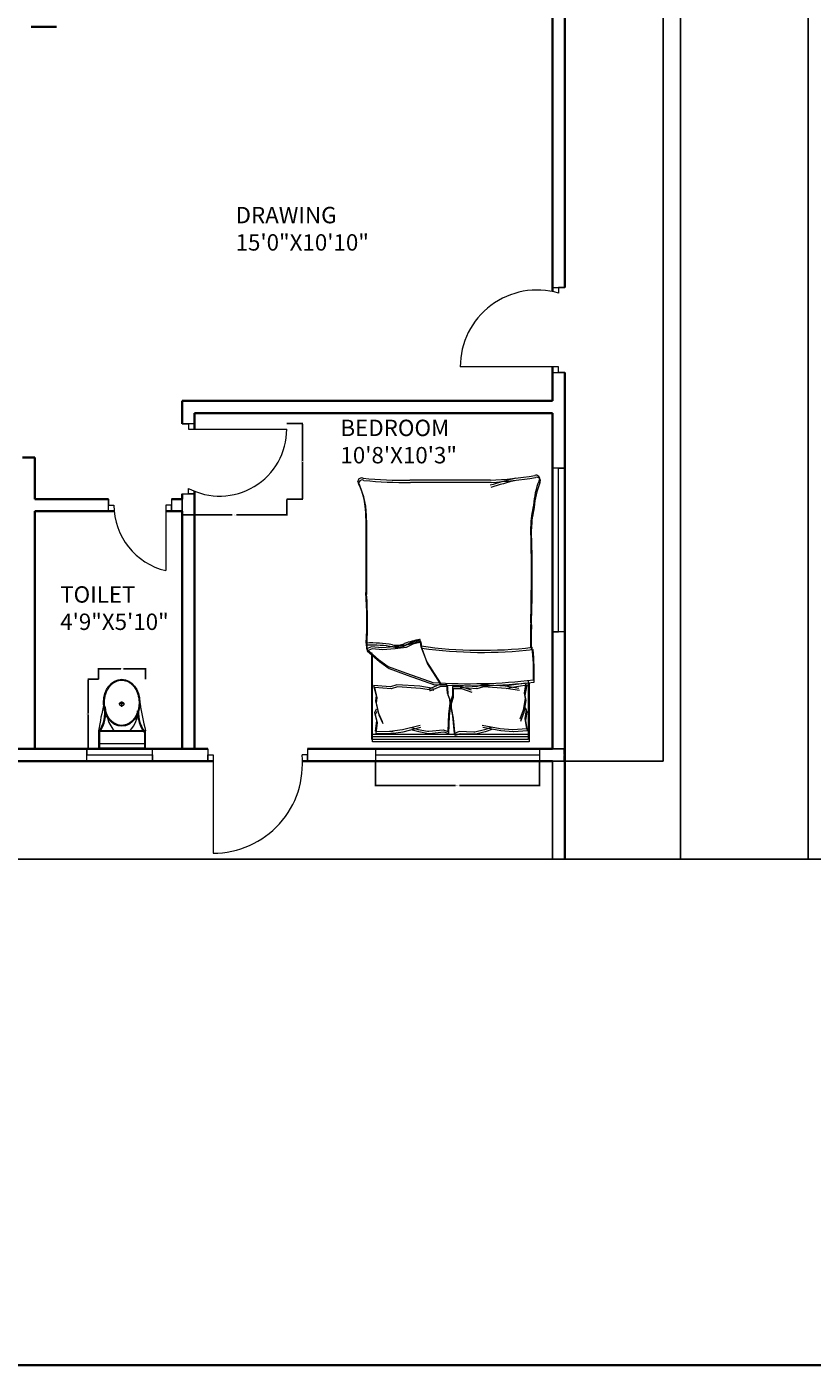
# Model space of a CAD drawing. Units: inches. Extents: x 1520 to 3401, y 1570 to 3432.
# Tile 3 of 15: x 2147 to 2435, y 1570 to 2061. Entities that reach past the tile are written whole.
import ezdxf

# ---------------------------------------------------------------- set-up
doc = ezdxf.new("R2010")
doc.units = ezdxf.units.IN
for name, color, linetype, lineweight in [('A-ANNO-DIMS', 2, 'Continuous', 18), ('A-ANNO-TTLB', 7, 'Continuous', 35), ('A-AREA-IDEN', 7, 'Continuous', 18), ('A-DOOR', 3, 'Continuous', 18), ('A-FLOR-EDGE', 7, 'Continuous', 25), ('A-FLOR-FIXT', 9, 'Continuous', 18), ('A-FURN', 8, 'Continuous', 13), ('A-GLAZ', 4, 'Continuous', 18), ('A-WALL', 7, 'Continuous', 35)]:
    doc.layers.add(name, color=color, linetype=linetype, lineweight=lineweight)
doc.styles.get("Standard").update_dxf_attribs({"font": 'arial.ttf'})
doc.dimstyles.get("Standard").update_dxf_attribs({"dimtxt": 0.18, "dimasz": 0.18, "dimexe": 0.18, "dimexo": 0.0625, "dimgap": 0.09, "dimtad": 0, "dimtih": 1, "dimtoh": 1, "dimdec": 4, "dimzin": 0, "dimdsep": 46, "dimtxsty": 'Standard', "dimcen": 0.09, "dimadec": 0, "dimazin": 0, "dimtfac": 1, "dimtdec": 4, "dimtofl": 0, "dimtmove": 0, "dimatfit": 3, "dimfxl": 1, "dimtolj": 1, "dimtzin": 0, "dimarcsym": 0})

# ---------------------------------------------------------------- blocks, each defined once
blk = doc.blocks.new('A$C31115884')
for p, q in [((283, 498), (223, 498)), ((258, 466), (258, 523)), ((0, 200), (0, 0)), ((520, 200), (0, 200)), ((10, 190), (10, 10)), ((510, 190), (10, 190)), ((510, 10), (510, 190)), ((520, 0), (520, 200)), ((510, 54), (0, 54)), ((10, 10), (510, 10)), ((0, 0), (520, 0))]:
    blk.add_line(p, q)
blk.add_circle((256, 496), 23.6)
for centre, radius, start, end in [((2778, -205), 2807, 165.4549, 171.7133), ((-295, 403), 365, 324.2091, 9.3499), ((-295, 403), 375, 324.2091, 9.3499), ((806, 403), 365, 170.6501, 215.7909), ((3237, 905), 2807, 188.2867, 194.5451), ((384, 406), 293, 190.2774, 224.1564), ((139, 406), 293, 315.8436, 2.6563), ((806, 403), 375, 179.2036, 215.7909)]:
    blk.add_arc(centre, radius, start, end)
blk.add_ellipse((256, 510), major_axis=(0, -261), ratio=0.772727)
blk.add_open_spline([(256, 259), (263, 259), (270, 260), (288, 262), (299, 265), (320, 273), (330, 278), (350, 291), (360, 299), (378, 316), (386, 326), (402, 347), (409, 358), (421, 383), (427, 395), (436, 422), (440, 436), (445, 465), (447, 480), (448, 509), (448, 524), (445, 553), (443, 568), (436, 596), (432, 610), (422, 636), (416, 649), (402, 672), (395, 683), (379, 703), (370, 712), (351, 728), (341, 735), (321, 746), (310, 751), (289, 757), (278, 759), (256, 761), (245, 761), (223, 757), (212, 754), (191, 746), (181, 741), (161, 728), (151, 720), (133, 703), (125, 693), (110, 672), (103, 660), (90, 636), (85, 623), (76, 596), (72, 582), (67, 553), (66, 538), (64, 509), (65, 494), (68, 465), (70, 450), (77, 422), (81, 408), (91, 382), (97, 370), (111, 346), (118, 335), (135, 316), (144, 307), (162, 291), (172, 284), (193, 273), (203, 269), (225, 262), (236, 260), (250, 259), (253, 259), (256, 259)], degree=3, knots=[0, 0, 0, 0, 0.110105, 0.110105, 0.285049, 0.285049, 0.459994, 0.459994, 0.634938, 0.634938, 0.809882, 0.809882, 0.984827, 0.984827, 1.159771, 1.159771, 1.334715, 1.334715, 1.50966, 1.50966, 1.684604, 1.684604, 1.859549, 1.859549, 2.034493, 2.034493, 2.209437, 2.209437, 2.384382, 2.384382, 2.559326, 2.559326, 2.73427, 2.73427, 2.909215, 2.909215, 3.084159, 3.084159, 3.259103, 3.259103, 3.434048, 3.434048, 3.608992, 3.608992, 3.783936, 3.783936, 3.958881, 3.958881, 4.133825, 4.133825, 4.30877, 4.30877, 4.483714, 4.483714, 4.658658, 4.658658, 4.833603, 4.833603, 5.008547, 5.008547, 5.183491, 5.183491, 5.358436, 5.358436, 5.53338, 5.53338, 5.708324, 5.708324, 5.883269, 5.883269, 6.058213, 6.058213, 6.233158, 6.233158, 6.283185, 6.283185, 6.283185, 6.283185])
blk = doc.blocks.new('DOOR-SWING-24-10')
for p, q in [((0, 21.75), (0, 26.25)), ((0, 26.25), (0, 24)), ((23.01, 26.25), (23.01, 21.75)), ((0, 24), (2, 24)), ((23.01, 24), (21.01, 24)), ((21.01, 24), (21.01, 0)), ((23.01, 21.75), (23.01, 24))]:
    blk.add_line(p, q)
blk.add_arc((26.65, 24), 24.65, 180, 256.7773)
blk = doc.blocks.new('DOOR-SWING-36-11')
for p, q in [((4.5, 26.53), (0, 26.53)), ((0, 26.53), (2.25, 26.53)), ((2.25, 26.53), (2.25, 24.53)), ((2.25, 24.53), (38.25, 24.53)), ((0, 0.83), (4.5, 0.83)), ((2.25, 0.83), (2.25, 2.83)), ((4.5, 0.83), (2.25, 0.83))]:
    blk.add_line(p, q)
blk.add_arc((13.71, 24.53), 24.54, 242.1673, 0)
blk = doc.blocks.new('DOOR-SWING-36-27')
for p, q in [((0, 38.25), (0, 33.75)), ((0, 33.75), (0, 36)), ((0, 36), (2, 36)), ((2, 36), (2, 0)), ((36.5, 36), (34.5, 36)), ((36.5, 38.25), (36.5, 33.75)), ((36.5, 33.75), (36.5, 36))]:
    blk.add_line(p, q)
blk.add_arc((2, 32.67), 32.67, 270, 5.849)
blk = doc.blocks.new('DOOR-SWING-36-30')
for p, q in [((33.75, 31.05), (38.25, 31.05)), ((38.25, 31.05), (36, 31.05)), ((36, 31.05), (36, 29.05)), ((36, 2), (0, 2)), ((33.75, 0), (38.25, 0)), ((36, 0), (36, 2)), ((38.25, 0), (36, 0))]:
    blk.add_line(p, q)
blk.add_arc((28.16, 2), 28.16, 73.8433, 180)
blk = doc.blocks.new('WIN-PLAN-24-01')
for p, q in [((0, 4.5), (0, 0)), ((0, 0), (0, 2.25)), ((0, 2.25), (24, 2.25)), ((24, 2.25), (24, 4.5)), ((24, 4.5), (24, 0))]:
    blk.add_line(p, q)
blk = doc.blocks.new('WIN-PLAN-60-02')
for p, q in [((4.5, 60), (0, 60)), ((0, 60), (2.25, 60)), ((2.25, 60), (2.25, 0)), ((4.5, 0), (0, 0)), ((2.25, 0), (4.5, 0))]:
    blk.add_line(p, q)
blk = doc.blocks.new('WIN-PLAN-60-05')
for p, q in [((0, 4.5), (0, 0)), ((0, 2.25), (60, 2.25)), ((60, 4.5), (60, 0))]:
    blk.add_line(p, q)
blk = doc.blocks.new('BED-DOUBLE')
for p, q in [((4.17, 75.93), (4.17, 97.64)), ((4.17, 97.64), (61.46, 97.64)), ((4.17, 95.8), (61.46, 95.8)), ((4.44, 75.16), (4.44, 96.87)), ((4.44, 96.87), (61.73, 96.87)), ((4.44, 95.03), (61.73, 95.03)), ((4.67, 93.64), (9.81, 94.03)), ((4.67, 93.66), (5.36, 89.85)), ((4.95, 92.87), (10.08, 93.27)), ((9.81, 94.03), (9.93, 94.01)), ((9.93, 94.01), (14.52, 93.66)), ((10.08, 93.27), (10.21, 93.24)), ((10.21, 93.24), (14.79, 92.9)), ((14.52, 93.66), (21.1, 92.45)), ((17.81, 93.14), (20.24, 94.01)), ((18.08, 92.38), (20.51, 93.24)), ((20.24, 94.01), (23.7, 94.88)), ((20.51, 93.24), (23.98, 94.11)), ((23.7, 94.88), (24.09, 94.88)), ((23.98, 94.11), (24.36, 94.11)), ((24.09, 94.88), (29.42, 94.7)), ((24.36, 94.11), (29.69, 93.94)), ((29.42, 94.7), (31.15, 95.4)), ((29.69, 93.94), (31.42, 94.63)), ((31.15, 95.4), (31.84, 88.98)), ((31.42, 94.63), (32.12, 88.22)), ((33.54, 94.65), (33.25, 88.21)), ((33.81, 93.88), (33.52, 87.44)), ((35.31, 94.07), (33.54, 94.65)), ((35.59, 93.3), (33.81, 93.88)), ((40.62, 94.57), (35.31, 94.07)), ((40.9, 93.81), (35.59, 93.3)), ((41.01, 94.6), (40.62, 94.57)), ((41.28, 93.83), (40.9, 93.81)), ((44.52, 93.95), (41.01, 94.6)), ((44.79, 93.18), (41.28, 93.83)), ((50.25, 93.96), (43.75, 92.34)), ((50.52, 93.19), (44.03, 91.57)), ((47, 93.23), (44.52, 93.95)), ((47.27, 92.47), (44.79, 93.18)), ((54.8, 94.59), (50.25, 93.96)), ((55.08, 93.82), (50.52, 93.19)), ((60.08, 94.57), (53.6, 94.69)), ((53.6, 94.69), (54.8, 94.59)), ((60.35, 93.81), (53.87, 93.92)), ((53.87, 93.92), (55.08, 93.82)), ((60.08, 94.57), (59.62, 90.72)), ((60.35, 93.81), (59.9, 89.96)), ((61.46, 97.64), (61.46, 65.74)), ((61.73, 96.87), (61.73, 64.97)), ((5.36, 89.85), (4.84, 86.73)), ((4.94, 92.9), (5.64, 89.08)), ((5.64, 89.08), (5.12, 85.96)), ((6.06, 86.9), (7.27, 90.2)), ((6.33, 86.14), (7.54, 89.43)), ((14.79, 92.9), (21.38, 91.68)), ((31.84, 88.98), (32.54, 85.17)), ((59.12, 87.74), (57.7, 90.95)), ((59.39, 86.97), (57.97, 90.18)), ((59.62, 90.72), (60.34, 87.64)), ((59.9, 89.96), (60.61, 86.88)), ((4.84, 86.73), (5.54, 85.52)), ((5.12, 85.96), (5.81, 84.75)), ((5.36, 82.57), (6.06, 86.9)), ((5.64, 81.8), (6.33, 86.14)), ((32.54, 83.61), (31.84, 81.36)), ((32.12, 88.22), (32.81, 84.4)), ((32.54, 85.17), (32.54, 83.61)), ((33.25, 88.21), (32.79, 84.36)), ((32.79, 84.36), (32.89, 82.8)), ((32.81, 84.4), (32.81, 82.84)), ((33.52, 87.44), (33.07, 83.59)), ((33.07, 83.59), (33.17, 82.03)), ((60.08, 83.46), (59.12, 87.74)), ((60.35, 82.69), (59.39, 86.97)), ((60.34, 87.64), (59.72, 86.39)), ((59.85, 81.53), (60.08, 83.46)), ((60.61, 86.88), (59.99, 85.62)), ((5.02, 76.85), (5.71, 80.66)), ((5.29, 76.08), (5.98, 79.9)), ((5.71, 80.66), (5.36, 82.57)), ((5.98, 79.9), (5.64, 81.8)), ((7.65, 78.9), (12.48, 78.1)), ((28.9, 78.14), (25.13, 79.45)), ((29.17, 77.37), (25.4, 78.68)), ((31.84, 81.36), (31.84, 78.14)), ((32.81, 82.84), (32.12, 80.59)), ((32.12, 80.59), (32.12, 77.37)), ((32.89, 82.8), (33.72, 80.59)), ((33.17, 82.03), (34, 79.83)), ((33.72, 80.59), (33.93, 77.39)), ((34, 79.83), (34.2, 76.62)), ((36.87, 77.57), (40.55, 79.11)), ((39.04, 78.9), (43.87, 78.1)), ((60.78, 77.77), (59.85, 81.53)), ((60.12, 80.77), (60.35, 82.69)), ((61.05, 77), (60.12, 80.77)), ((11.13, 77.72), (5.02, 76.85)), ((11.4, 76.95), (5.29, 76.08)), ((7.92, 78.14), (12.76, 77.34)), ((12.48, 78.1), (11.13, 77.72)), ((12.76, 77.34), (11.4, 76.95)), ((12.48, 78.1), (20.89, 77.59)), ((12.76, 77.34), (21.16, 76.82)), ((20.89, 77.59), (23.24, 78.25)), ((21.16, 76.82), (23.51, 77.49)), ((23.24, 78.25), (29.39, 77.77)), ((23.51, 77.49), (29.67, 77)), ((31.84, 78.14), (28.9, 78.14)), ((32.12, 77.37), (29.17, 77.37)), ((33.93, 77.39), (36.87, 77.57)), ((34.2, 76.62), (37.14, 76.8)), ((36.28, 76.8), (41.3, 69.01)), ((36.55, 76.03), (41.57, 68.25)), ((37.14, 76.8), (40.82, 78.34)), ((48.73, 73.28), (38.73, 76.8)), ((49, 72.52), (39, 76.03)), ((39.31, 78.14), (44.15, 77.34)), ((43.87, 78.1), (52.28, 77.59)), ((44.15, 77.34), (52.55, 76.82)), ((52.28, 77.59), (54.63, 78.25)), ((52.55, 76.82), (54.9, 77.49)), ((54.63, 78.25), (60.78, 77.77)), ((54.9, 77.49), (61.05, 77)), ((41.3, 69.01), (43.34, 63.63)), ((55.41, 70.87), (48.73, 73.28)), ((55.69, 70.1), (49, 72.52)), ((58.94, 68.27), (55.41, 70.87)), ((59.21, 67.51), (55.69, 70.1)), ((41.57, 68.25), (43.62, 62.87)), ((53.18, 63.63), (57.82, 64)), ((57.82, 64), (61.54, 63.63)), ((63.38, 64.38), (58.94, 68.27)), ((63.66, 63.61), (59.21, 67.51)), ((61.54, 63.63), (63.38, 64.38)), ((63.48, 62.28), (63.38, 64.38, 4.64)), ((43.34, 63.63), (43.71, 61.22)), ((43.62, 62.87), (43.99, 60.45)), ((43.71, 61.22), (46.68, 61.96)), ((43.99, 60.45), (46.96, 61.2)), ((46.68, 61.96), (49.1, 63.08)), ((46.96, 61.2), (49.37, 62.31)), ((49.1, 63.08), (53.18, 63.63)), ((49.37, 62.31), (53.46, 62.87)), ((53.46, 62.87), (58.1, 63.24)), ((58.1, 63.24), (61.81, 62.87)), ((61.81, 62.87), (63.66, 63.61)), ((63.75, 61.52), (63.66, 63.61, 4.64)), ((18.06, 2.64), (47.57, 2.64)), ((18.33, 1.87), (47.84, 1.87))]:
    blk.add_line(p, q)
for centre, radius, start, end in [((102.1, 73.55), 99.87, 178.7218, 185.604), ((25.61, -120.62), 197.77, 86.0865, 96.7821), ((102.37, 72.78), 99.87, 178.7218, 185.604), ((25.88, -121.38), 197.77, 86.0865, 96.7821), ((21.29, -89.76), 154.68, 81.7845, 96.9006), ((21.56, -90.53), 154.68, 81.7845, 96.9006), ((-200.58, 60.27), 203.94, 358.4762, 1.0082), ((-200.3, 59.5), 203.94, 358.4762, 1.0082), ((43.92, 61.15), 0.221, 160.2464, 271.1377), ((37.35, 95.86), 35.55, 280.6617, 289.8806), ((44.2, 60.38), 0.221, 160.2464, 271.1377), ((37.62, 95.1), 35.55, 280.6617, 289.8806), ((52.44, 55.6), 7.46, 78.6608, 113.7384), ((52.72, 54.83), 7.46, 78.6608, 113.7384), ((61.53, 105.62), 43.38, 259.8763, 272.5657), ((61.81, 104.85), 43.38, 259.8763, 272.5657), ((218.51, 54.1), 155.25, 176.9791, 183.8365), ((218.79, 53.34), 155.25, 176.9791, 183.8365), ((581.23, 36.96), 578.22, 178.22771, 181.71854), ((581.51, 36.19), 578.22, 178.22771, 181.71854), ((-5405.34, 16.33), 5469.02, 0.00217, 0.28689), ((-5405.07, 15.56), 5469.02, 0.00217, 0.28689), ((-32.25, 20.29), 35.53, 346.0648, 358.9113), ((-31.97, 19.53), 35.53, 346.0648, 358.9113), ((91.3, 15.32), 27.65, 177.4714, 206.4681), ((91.58, 14.55), 27.65, 177.4714, 206.4681), ((-25.97, 13.39), 28.25, 337.9751, 356.652), ((-25.69, 12.62), 28.25, 337.9751, 356.652), ((1.3, 2.07), 1.31, 146.1736, 293.4781), ((1.58, 1.3), 1.31, 146.1736, 293.4781), ((25.69, -143.14), 145.97, 92.9958, 99.4091), ((25.96, -143.9), 145.97, 92.9958, 99.4091), ((-20.65, 126.07), 127.63, 283.3832, 287.7053), ((-20.37, 125.3), 127.63, 283.3832, 287.7053), ((49.34, -156.85), 159.5, 84.4998, 90.6351), ((49.61, -157.62), 159.5, 84.4998, 90.6351), ((65.23, 3.08), 1.32, 242.6588, 356.02), ((65.5, 2.32), 1.32, 242.6588, 356.02)]:
    blk.add_arc(centre, radius, start, end)
blk = doc.blocks.new('*D67')
at = {"layer": 'A-ANNO-DIMS', "color": 0, "lineweight": -2, "transparency": 16777216}
for p, q in [((2173.44, 1821.66), (2169.5, 1821.66)), ((2169.68, 1821.48), (2169.68, 1809.1)), ((2169.68, 1796.36), (2169.68, 1808.73)), ((2173.44, 1796.18), (2169.5, 1796.18))]:
    blk.add_line(p, q, dxfattribs=at)
at = {"layer": 'A-ANNO-DIMS', "color": 0, "transparency": 16777216}
for points in [[(2169.65, 1821.48), (2169.71, 1821.48), (2169.68, 1821.66)], [(2169.65, 1796.36), (2169.71, 1796.36), (2169.68, 1796.18)]]:
    blk.add_solid(points, dxfattribs=at)
at = {"layer": 'Defpoints', "color": 0, "transparency": 16777216}
for p in [(2169.68, 1821.66), (2173.5, 1821.66), (2173.5, 1796.18)]:
    blk.add_point(p, dxfattribs=at)
at = {"layer": 'A-ANNO-DIMS', "color": 0, "transparency": 16777216, "insert": (2169.68, 1808.92), "char_height": 0.18, "attachment_point": 5}
blk.add_mtext('\\A1;WC 25 TYP.', dxfattribs=at)
blk = doc.blocks.new('*D68')
at = {"layer": 'A-ANNO-DIMS', "color": 0, "lineweight": -2, "transparency": 16777216}
for p, q in [((2173.5, 1821.72), (2173.5, 1825.66)), ((2173.68, 1825.48), (2181.58, 1825.48)), ((2190.51, 1825.48), (2182.62, 1825.48)), ((2190.69, 1821.72), (2190.69, 1825.66))]:
    blk.add_line(p, q, dxfattribs=at)
at = {"layer": 'A-ANNO-DIMS', "color": 0, "transparency": 16777216}
for points in [[(2173.68, 1825.51), (2173.68, 1825.45), (2173.5, 1825.48)], [(2190.51, 1825.51), (2190.51, 1825.45), (2190.69, 1825.48)]]:
    blk.add_solid(points, dxfattribs=at)
at = {"layer": 'Defpoints', "color": 0, "transparency": 16777216}
for p in [(2190.69, 1825.48), (2173.5, 1821.66), (2190.69, 1821.66)]:
    blk.add_point(p, dxfattribs=at)
at = {"layer": 'A-ANNO-DIMS', "color": 0, "transparency": 16777216, "insert": (2182.1, 1825.48), "char_height": 0.18, "attachment_point": 5}
blk.add_mtext('\\A1;17 TYP.', dxfattribs=at)
blk = doc.blocks.new('*D101')
at = {"layer": 'A-ANNO-DIMS', "color": 0, "lineweight": -2, "transparency": 16777216}
for p, q in [((2204.11, 1887.49), (2204.11, 1881.64)), ((2242.36, 1887.49), (2242.36, 1881.64)), ((2204.29, 1881.82), (2222.45, 1881.82)), ((2242.18, 1881.82), (2224.03, 1881.82))]:
    blk.add_line(p, q, dxfattribs=at)
at = {"layer": 'A-ANNO-DIMS', "color": 0, "transparency": 16777216}
for points in [[(2204.29, 1881.85), (2204.29, 1881.79), (2204.11, 1881.82)], [(2242.18, 1881.85), (2242.18, 1881.79), (2242.36, 1881.82)]]:
    blk.add_solid(points, dxfattribs=at)
at = {"layer": 'Defpoints', "color": 0, "transparency": 16777216}
for p in [(2204.11, 1887.56), (2242.36, 1887.56), (2242.36, 1881.82)]:
    blk.add_point(p, dxfattribs=at)
at = {"layer": 'A-ANNO-DIMS', "color": 0, "transparency": 16777216, "insert": (2223.24, 1881.82), "char_height": 0.18, "attachment_point": 5}
blk.add_mtext('\\A1;D11 38 TYP.', dxfattribs=at)
blk = doc.blocks.new('*D102')
at = {"layer": 'A-ANNO-DIMS', "color": 0, "lineweight": -2, "transparency": 16777216}
for p, q in [((2242.43, 1915.28), (2248.28, 1915.28)), ((2248.1, 1915.1), (2248.1, 1901.6)), ((2248.1, 1887.74), (2248.1, 1901.23)), ((2242.43, 1887.56), (2248.28, 1887.56))]:
    blk.add_line(p, q, dxfattribs=at)
at = {"layer": 'A-ANNO-DIMS', "color": 0, "transparency": 16777216}
for points in [[(2248.07, 1915.1), (2248.13, 1915.1), (2248.1, 1915.28)], [(2248.07, 1887.74), (2248.13, 1887.74), (2248.1, 1887.56)]]:
    blk.add_solid(points, dxfattribs=at)
at = {"layer": 'Defpoints', "color": 0, "transparency": 16777216}
for p in [(2242.36, 1915.28), (2248.1, 1915.28), (2242.36, 1887.56)]:
    blk.add_point(p, dxfattribs=at)
at = {"layer": 'A-ANNO-DIMS', "color": 0, "transparency": 16777216, "insert": (2248.1, 1901.42), "char_height": 0.18, "attachment_point": 5}
blk.add_mtext('\\A1;28 TYP.', dxfattribs=at)
blk = doc.blocks.new('*D141')
at = {"layer": 'A-ANNO-DIMS', "color": 0, "lineweight": -2, "transparency": 16777216}
for p, q in [((2274.88, 1791.62), (2274.88, 1782.5)), ((2334.88, 1791.62), (2334.88, 1782.5)), ((2275.06, 1782.68), (2304.13, 1782.68)), ((2334.7, 1782.68), (2305.64, 1782.68))]:
    blk.add_line(p, q, dxfattribs=at)
at = {"layer": 'A-ANNO-DIMS', "color": 0, "transparency": 16777216}
for points in [[(2275.06, 1782.71), (2275.06, 1782.65), (2274.88, 1782.68)], [(2334.7, 1782.71), (2334.7, 1782.65), (2334.88, 1782.68)]]:
    blk.add_solid(points, dxfattribs=at)
at = {"layer": 'Defpoints', "color": 0, "transparency": 16777216}
for p in [(2274.88, 1791.68), (2334.88, 1791.68), (2334.88, 1782.68)]:
    blk.add_point(p, dxfattribs=at)
at = {"layer": 'A-ANNO-DIMS', "color": 0, "transparency": 16777216, "insert": (2304.88, 1782.68), "char_height": 0.18, "attachment_point": 5}
blk.add_mtext('\\A1;W5 60 TYP.', dxfattribs=at)
blk = doc.blocks.new('*D142')
at = {"layer": 'A-ANNO-DIMS', "color": 0, "lineweight": -2, "transparency": 16777216}
for p, q in [((2334.95, 1796.18), (2344.06, 1796.18)), ((2343.88, 1796), (2343.88, 1794.11)), ((2334.95, 1791.68), (2344.06, 1791.68)), ((2343.88, 1791.86), (2343.88, 1793.75))]:
    blk.add_line(p, q, dxfattribs=at)
at = {"layer": 'A-ANNO-DIMS', "color": 0, "transparency": 16777216}
for points in [[(2343.85, 1796), (2343.91, 1796), (2343.88, 1796.18)], [(2343.85, 1791.86), (2343.91, 1791.86), (2343.88, 1791.68)]]:
    blk.add_solid(points, dxfattribs=at)
at = {"layer": 'Defpoints', "color": 0, "transparency": 16777216}
for p in [(2334.88, 1796.18), (2343.88, 1796.18), (2334.88, 1791.68)]:
    blk.add_point(p, dxfattribs=at)
at = {"layer": 'A-ANNO-DIMS', "color": 0, "transparency": 16777216, "insert": (2343.88, 1793.93), "char_height": 0.18, "attachment_point": 5}
blk.add_mtext('\\A1;5 TYP.', dxfattribs=at)
blk = doc.blocks.new('*D182')
at = {"layer": 'A-ANNO-DIMS', "color": 0, "lineweight": -2, "transparency": 16777216}
for p, q in [((2380.18, 2733.18), (2433.39, 2733.18)), ((2433.21, 2733), (2433.21, 2244.61)), ((2433.21, 1755.86), (2433.21, 2244.25)), ((2344.18, 1755.68), (2433.39, 1755.68))]:
    blk.add_line(p, q, dxfattribs=at)
at = {"layer": 'A-ANNO-DIMS', "color": 0, "transparency": 16777216}
for points in [[(2433.18, 2733), (2433.24, 2733), (2433.21, 2733.18)], [(2433.18, 1755.86), (2433.24, 1755.86), (2433.21, 1755.68)]]:
    blk.add_solid(points, dxfattribs=at)
at = {"layer": 'Defpoints', "color": 0, "transparency": 16777216}
for p in [(2380.11, 2733.18), (2344.11, 1755.68), (2433.21, 1755.68)]:
    blk.add_point(p, dxfattribs=at)
at = {"layer": 'A-ANNO-DIMS', "color": 0, "transparency": 16777216, "insert": (2433.21, 2244.43), "char_height": 0.18, "attachment_point": 5}
blk.add_mtext('\\A1;977.5', dxfattribs=at)
blk = doc.blocks.new('*D192')
at = {"layer": 'A-ANNO-DIMS', "color": 0, "lineweight": -2, "transparency": 16777216}
for p, q in [((2467.84, 2733.18), (2386.32, 2733.18)), ((2386.5, 2733), (2386.5, 2244.61)), ((2386.5, 1755.86), (2386.5, 2244.25)), ((2503.84, 1755.68), (2386.32, 1755.68))]:
    blk.add_line(p, q, dxfattribs=at)
at = {"layer": 'A-ANNO-DIMS', "color": 0, "transparency": 16777216}
for points in [[(2386.47, 2733), (2386.53, 2733), (2386.5, 2733.18)], [(2386.47, 1755.86), (2386.53, 1755.86), (2386.5, 1755.68)]]:
    blk.add_solid(points, dxfattribs=at)
at = {"layer": 'Defpoints', "color": 0, "transparency": 16777216}
for p in [(2467.9, 2733.18), (2386.5, 1755.68), (2503.9, 1755.68)]:
    blk.add_point(p, dxfattribs=at)
at = {"layer": 'A-ANNO-DIMS', "color": 0, "transparency": 16777216, "insert": (2386.5, 2244.43), "char_height": 0.18, "attachment_point": 5}
blk.add_mtext('\\A1;977.5', dxfattribs=at)

msp = doc.modelspace()

# ---------------------------------------------------------------- linework, layer by layer
at = {"layer": 'A-ANNO-TTLB'}
msp.add_lwpolyline([(1519.9253, 3431.7421), (3400.8761, 3431.7421), (3400.8761, 1570.3458), (1519.9253, 1570.3458)], close=True, dxfattribs=at)
at = {"layer": 'A-FLOR-EDGE'}
for p, q in [((2380.1128, 2733.1786), (2380.1128, 1791.6786)), ((2339.6128, 1791.6786), (2339.6128, 1755.6786)), ((2344.1128, 1791.6786), (2380.1128, 1791.6786)), ((1699.6128, 1755.6786), (2339.6128, 1755.6786)), ((2339.6128, 1755.6786), (2344.1128, 1755.6786))]:
    msp.add_line(p, q, dxfattribs=at)
at = {"layer": 'A-WALL'}
for p, q in [((2344.1128, 2432.7197), (2344.1128, 1965.1342)), ((2339.6128, 2431.1873), (2339.6128, 1963.6868)), ((2158.1128, 2060.6786), (2148.8169, 2060.6786)), ((2148.8169, 2060.6786), (2153.6128, 2060.6786)), ((2339.6128, 1936.0834), (2339.6128, 1923.6786)), ((2344.1128, 1934.0834), (2344.1128, 1755.6786)), ((2204.1128, 1923.6786), (2339.6128, 1923.6786)), ((2204.1128, 1915.2759), (2204.1128, 1923.6786)), ((2339.6128, 1919.1786), (2208.6128, 1919.1786)), ((2208.6128, 1919.1786), (2208.6128, 1913.2759)), ((2339.6128, 1919.1786), (2339.6128, 1796.1786)), ((2150.1128, 1902.917), (2145.6128, 1902.917)), ((2150.1128, 1887.6786), (2150.1128, 1902.917)), ((2204.1128, 1887.6786), (2204.1128, 1889.5733)), ((2208.6128, 1890.5272), (2208.6128, 1887.6786)), ((2177.1128, 1887.6786), (2150.1128, 1887.6786)), ((2150.1128, 1796.1786), (2150.1128, 1883.1786)), ((2179.2157, 1883.1786), (2150.1128, 1883.1786)), ((2204.1128, 1883.1786), (2198.1272, 1883.1786)), ((2204.1128, 1887.6786), (2200.1272, 1887.6786)), ((2204.1128, 1796.1786), (2204.1128, 1883.1786)), ((2208.6128, 1887.6786), (2208.6128, 1796.1786)), ((2213.4538, 1796.1786), (2139.1737, 1796.1786)), ((2145.6128, 1796.1786), (2150.1128, 1796.1786)), ((2150.1128, 1796.1786), (2204.1128, 1796.1786)), ((2339.6128, 1796.1786), (2249.9544, 1796.1786)), ((2215.4538, 1791.6786), (2137.1737, 1791.6786)), ((2339.6128, 1791.6786), (2248.1066, 1791.6786))]:
    msp.add_line(p, q, dxfattribs=at)

# ---------------------------------------------------------------- block references
at = {"layer": 'A-DOOR'}
for name, p in [('DOOR-SWING-36-30', (2305.863, 1934.083)), ('DOOR-SWING-36-11', (2204.113, 1888.744)), ('DOOR-SWING-24-10', (2177.113, 1861.429)), ('DOOR-SWING-36-27', (2213.454, 1757.929))]:
    msp.add_blockref(name, p, dxfattribs=at)
at = {"layer": 'A-FLOR-FIXT', "xscale": 0.0330640103915726, "yscale": 0.0330640103915726, "zscale": 0.0330640103915726}
msp.add_blockref('A$C31115884', (2173.5, 1796.1786), dxfattribs=at)
at = {"layer": 'A-FURN', "rotation": 180}
msp.add_blockref('BED-DOUBLE', (2335.2231, 1896.4054), dxfattribs=at)
at = {"layer": 'A-GLAZ', "extrusion": (0, 0, -1), "zscale": -1, "rotation": 180}
for name, p in [('WIN-PLAN-60-02', (-2339.613, 1898.9765)), ('WIN-PLAN-24-01', (-2169.2275, 1796.1783))]:
    msp.add_blockref(name, p, dxfattribs=at)
at = {"layer": 'A-GLAZ'}
msp.add_blockref('WIN-PLAN-60-05', (2274.885, 1791.679), dxfattribs=at)

# ---------------------------------------------------------------- texts
at = {"layer": 'A-AREA-IDEN', "char_height": 6, "attachment_point": 1}
for s, width, insert in [('DRAWING\\P15\'0"X10\'10"', 87.593209, (2223.6418, 1994.6865)), ('BEDROOM\\P10\'8\'X10\'3"', 113.7935, (2262.018, 1916.7348)), ('TOILET\\P4\'9"X5\'10"', 75.838771, (2159.4432, 1855.7102))]:
    msp.add_mtext_dynamic_manual_height_columns(s, width=width, gutter_width=12.5, heights=[0], dxfattribs=dict(at, insert=insert))

# ---------------------------------------------------------------- dimensions: what is measured, and where the dimension line sits
at = {"layer": 'A-ANNO-DIMS'}
for base, p1, p2, picture, middle in [((2433.2128, 1755.6786), (2380.1128, 2733.1786), (2344.1128, 1755.6786), '*D182', (2433.2128, 2244.4286)), ((2386.4982, 1755.6786), (2467.8987, 2733.1786), (2503.8987, 1755.6786), '*D192', (2386.4982, 2244.4286))]:
    dim = msp.add_linear_dim(base=base, p1=p1, p2=p2, angle=90, dimstyle='Standard', override={"dimdec": 1, "dimlfac": 1, "dimrnd": 0, "dimzin": 0, "dimdsep": 46, "dimlunit": 2}, dxfattribs=at)
    dim.commit()
    dim.dimension.update_dxf_attribs({"geometry": picture, "text_midpoint": middle})
for base, p1, p2, text, picture, middle in [((2248.1003, 1915.2759), (2242.3628, 1887.557), (2242.3628, 1915.2759), '<> TYP.', '*D102', (2248.1003, 1901.4164)), ((2169.6783, 1821.6568), (2173.5, 1796.1786), (2173.5, 1821.6568), 'WC <> TYP.', '*D67', (2169.6783, 1808.9177)), ((2343.8849805529, 1796.1786294992), (2334.8849805529, 1791.6786294992), (2334.8849805529, 1796.1786294992), '<> TYP.', '*D142', (2343.8849805529, 1793.9286294992))]:
    dim = msp.add_linear_dim(base=base, p1=p1, p2=p2, angle=90, text=text, dimstyle='Standard', override={"dimdec": 0, "dimlfac": 1, "dimrnd": 0, "dimzin": 0, "dimdsep": 46, "dimlunit": 2}, dxfattribs=at)
    dim.commit()
    dim.dimension.update_dxf_attribs({"geometry": picture, "text_midpoint": middle})
for base, p1, p2, text, picture, middle in [((2242.3628, 1881.8195), (2204.1128, 1887.557), (2242.3628, 1887.557), 'D11 <> TYP.', '*D101', (2223.2378, 1881.8195)), ((2190.6933, 1825.4785), (2173.5, 1821.6568), (2190.6933, 1821.6568), '<> TYP.', '*D68', (2182.0966, 1825.4785)), ((2334.885, 1782.6786), (2274.885, 1791.6786), (2334.885, 1791.6786), 'W5 <> TYP.', '*D141', (2304.885, 1782.6786))]:
    dim = msp.add_linear_dim(base=base, p1=p1, p2=p2, text=text, dimstyle='Standard', override={"dimdec": 0, "dimlfac": 1, "dimrnd": 0, "dimzin": 0, "dimdsep": 46, "dimlunit": 2}, dxfattribs=at)
    dim.commit()
    dim.dimension.update_dxf_attribs({"geometry": picture, "text_midpoint": middle})

doc.saveas('drawing.dxf')
